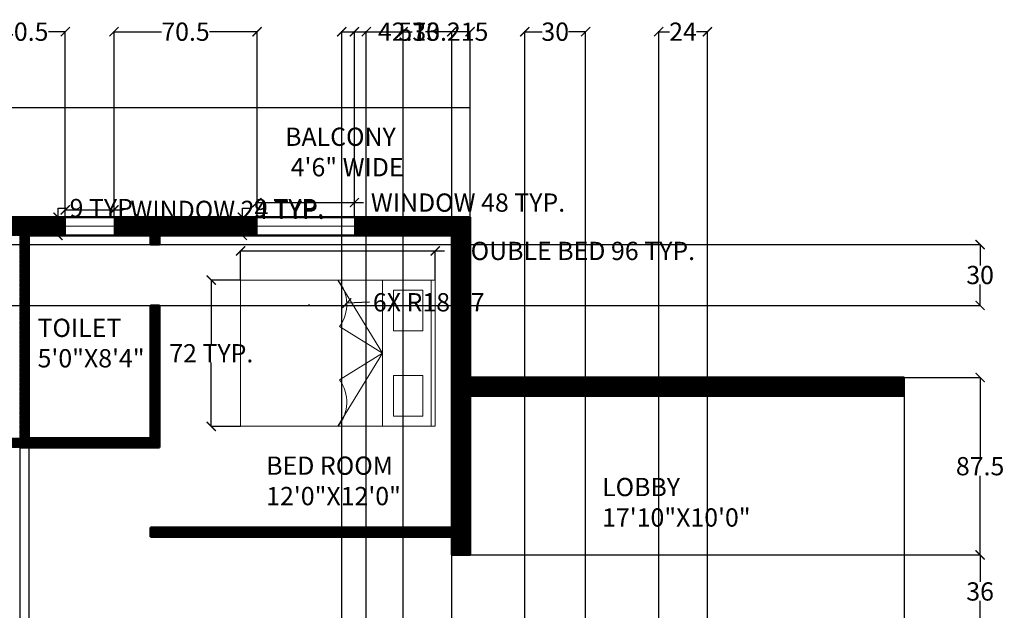
# Model space of a CAD drawing. Units: inches. Extents: x 273 to 1105, y 406 to 1027.
# Tile 3 of 3: x 612 to 1098, y 736 to 1027. Entities that reach past the tile are written whole.
import ezdxf

# ---------------------------------------------------------------- set-up
doc = ezdxf.new("R2010")
doc.units = ezdxf.units.IN
doc.header["$MEASUREMENT"] = 0
for name, color, linetype, lineweight in [('A-ANNO-DIMS', 2, 'Continuous', 18), ('A-AREA-IDEN', 7, 'Continuous', 18), ('A-FLOR-OTLN', 7, 'Continuous', 25), ('A-FURN', 8, 'Continuous', 18), ('A-GLAZ', 4, 'Continuous', 18), ('A-WALL', 7, 'Continuous', 50), ('A-WALL-PATT', 252, 'Continuous', 13)]:
    doc.layers.add(name, color=color, linetype=linetype, lineweight=lineweight)
doc.styles.get("Standard").update_dxf_attribs({"font": 'arial.ttf'})
doc.dimstyles.get("Standard").update_dxf_attribs({"dimtxt": 9, "dimasz": 4.5, "dimexe": 0.18, "dimexo": 0.0625, "dimgap": 0.09, "dimtad": 0, "dimtih": 1, "dimtoh": 1, "dimdec": 1, "dimzin": 0, "dimdsep": 46, "dimlunit": 4, "dimtxsty": 'Standard', "dimblk": 'ARCHTICK', "dimcen": 0.09, "dimadec": 0, "dimazin": 0, "dimtfac": 1, "dimtdec": 1, "dimtofl": 0, "dimtmove": 0, "dimatfit": 3, "dimfxl": 1, "dimtolj": 1, "dimtzin": 0, "dimarcsym": 0})

# ---------------------------------------------------------------- blocks, each defined once
blk = doc.blocks.new('BED-DOUBLE-72x96')
for p, q in [((0, 0.12), (0, 72.12)), ((0, 72.12), (96, 72.12)), ((48, 72.12), (70, 36.12)), ((70, 72.12), (70, 0.12)), ((94, 72.12), (94, 0.12)), ((96, 72.12), (96, 0.12)), ((48.84, 49.19), (70, 36.12)), ((70, 36.12), (48, 0.12)), ((70, 36.12), (48.84, 22.93)), ((96, 0.12), (0, 0.12))]:
    blk.add_line(p, q)
for points in [[(75.45, 67.24), (89.85, 67.24), (89.85, 47.07), (75.45, 47.07)], [(75.45, 5), (89.85, 5), (89.85, 25.18), (75.45, 25.18)]]:
    blk.add_lwpolyline(points, close=True)
for centre, start, end in [((33.83, 60.12), 323.9297, 40.2519), ((33.83, 12), 319.7481, 36.0703)]:
    blk.add_arc(centre, 18.57, start, end)
blk = doc.blocks.new('WIN-48')
for p, q in [((0, 9), (48, 9)), ((0, 0), (0, 9)), ((48, 9), (48, 0)), ((0, 4.5), (48, 4.5)), ((48, 0), (0, 0))]:
    blk.add_line(p, q)
blk = doc.blocks.new('WIN-24')
for p, q in [((0, 9), (24, 9)), ((0, 0), (0, 9)), ((24, 9), (24, 0)), ((0, 4.5), (24, 4.5)), ((24, 0), (0, 0))]:
    blk.add_line(p, q)
blk = doc.blocks.new('_ArchTick')
at = {"color": 0, "linetype": 'ByBlock', "const_width": 0.15}
blk.add_lwpolyline([(-0.5, -0.5), (0.5, 0.5)], dxfattribs=at)
blk = doc.blocks.new('*D6')
at = {"layer": 'A-ANNO-DIMS', "color": 0, "lineweight": -2, "transparency": 16777216}
for p, q in [((721.23, 898.64), (721.23, 913.15)), ((721.23, 912.97), (817.23, 912.97)), ((817.23, 898.64), (817.23, 913.15)), ((817.23, 912.97), (821.73, 912.97))]:
    blk.add_line(p, q, dxfattribs=at)
at = {"layer": 'Defpoints', "color": 0, "transparency": 16777216}
for p in [(817.23, 912.97), (721.23, 898.57), (817.23, 898.57)]:
    blk.add_point(p, dxfattribs=at)
at = {"layer": 'A-ANNO-DIMS', "color": 0, "lineweight": -2, "transparency": 16777216, "xscale": 4.5, "yscale": 4.5, "zscale": 4.5, "rotation": 180}
blk.add_blockref('_ArchTick', (721.23, 912.97), dxfattribs=at)
at = {"layer": 'A-ANNO-DIMS', "color": 0, "lineweight": -2, "transparency": 16777216, "xscale": 4.5, "yscale": 4.5, "zscale": 4.5}
blk.add_blockref('_ArchTick', (817.23, 912.97), dxfattribs=at)
at = {"layer": 'A-ANNO-DIMS', "color": 0, "transparency": 16777216, "insert": (885.77, 912.97), "char_height": 9, "attachment_point": 5}
blk.add_mtext('\\A1;DOUBLE BED 96 TYP.', dxfattribs=at)
blk = doc.blocks.new('*D7')
at = {"layer": 'A-ANNO-DIMS', "color": 0, "lineweight": -2, "transparency": 16777216}
for p, q in [((721.17, 898.57), (706.65, 898.57)), ((706.83, 898.57), (706.83, 867.12)), ((706.83, 826.45), (706.83, 857.9)), ((721.17, 826.45), (706.65, 826.45))]:
    blk.add_line(p, q, dxfattribs=at)
at = {"layer": 'Defpoints', "color": 0, "transparency": 16777216}
for p in [(706.83, 898.57), (721.23, 898.57), (721.23, 826.45)]:
    blk.add_point(p, dxfattribs=at)
at = {"layer": 'A-ANNO-DIMS', "color": 0, "lineweight": -2, "transparency": 16777216, "xscale": 4.5, "yscale": 4.5, "zscale": 4.5}
for p, rotation in [((706.83, 898.57), 90), ((706.83, 826.45), 270)]:
    blk.add_blockref('_ArchTick', p, dxfattribs=dict(at, rotation=rotation))
at = {"layer": 'A-ANNO-DIMS', "color": 0, "transparency": 16777216, "insert": (706.83, 862.51), "char_height": 9, "attachment_point": 5}
blk.add_mtext('\\A1;72 TYP.', dxfattribs=at)
blk = doc.blocks.new('*D8')
at = {"layer": 'A-ANNO-DIMS', "color": 0, "lineweight": -2, "transparency": 16777216}
for p, q in [((729.37, 929.67), (729.37, 936.98)), ((729.37, 936.8), (777.37, 936.8)), ((777.37, 929.67), (777.37, 936.98)), ((777.37, 936.8), (781.87, 936.8))]:
    blk.add_line(p, q, dxfattribs=at)
at = {"layer": 'Defpoints', "color": 0, "transparency": 16777216}
for p in [(777.37, 936.8), (729.37, 929.6), (777.37, 929.6)]:
    blk.add_point(p, dxfattribs=at)
at = {"layer": 'A-ANNO-DIMS', "color": 0, "lineweight": -2, "transparency": 16777216, "xscale": 4.5, "yscale": 4.5, "zscale": 4.5, "rotation": 180}
blk.add_blockref('_ArchTick', (729.37, 936.8), dxfattribs=at)
at = {"layer": 'A-ANNO-DIMS', "color": 0, "lineweight": -2, "transparency": 16777216, "xscale": 4.5, "yscale": 4.5, "zscale": 4.5}
blk.add_blockref('_ArchTick', (777.37, 936.8), dxfattribs=at)
at = {"layer": 'A-ANNO-DIMS', "color": 0, "transparency": 16777216, "insert": (833.38, 936.8), "char_height": 9, "attachment_point": 5}
blk.add_mtext('\\A1;WINDOW 48 TYP.', dxfattribs=at)
blk = doc.blocks.new('*D9')
at = {"layer": 'A-ANNO-DIMS', "color": 0, "lineweight": -2, "transparency": 16777216}
for p, q in [((722.17, 929.6), (722.17, 934.1)), ((722.17, 934.1), (726.67, 934.1)), ((729.31, 929.6), (721.99, 929.6)), ((722.17, 920.6), (722.17, 929.6)), ((729.31, 920.6), (721.99, 920.6))]:
    blk.add_line(p, q, dxfattribs=at)
at = {"layer": 'Defpoints', "color": 0, "transparency": 16777216}
for p in [(722.17, 929.6), (729.37, 929.6), (729.37, 920.6)]:
    blk.add_point(p, dxfattribs=at)
at = {"layer": 'A-ANNO-DIMS', "color": 0, "lineweight": -2, "transparency": 16777216, "xscale": 4.5, "yscale": 4.5, "zscale": 4.5}
for p, rotation in [((722.17, 929.6), 90), ((722.17, 920.6), 270)]:
    blk.add_blockref('_ArchTick', p, dxfattribs=dict(at, rotation=rotation))
at = {"layer": 'A-ANNO-DIMS', "color": 0, "transparency": 16777216, "insert": (745.17, 934.1), "char_height": 9, "attachment_point": 5}
blk.add_mtext('\\A1;9 TYP.', dxfattribs=at)
blk = doc.blocks.new('*D10')
at = {"layer": 'A-ANNO-DIMS', "color": 0, "lineweight": -2, "transparency": 16777216}
for p, q in [((634.87, 929.67), (634.87, 933.38)), ((634.87, 933.2), (658.87, 933.2)), ((658.87, 929.67), (658.87, 933.38)), ((658.87, 933.2), (663.37, 933.2))]:
    blk.add_line(p, q, dxfattribs=at)
at = {"layer": 'Defpoints', "color": 0, "transparency": 16777216}
for p in [(658.87, 933.2), (634.87, 929.6), (658.87, 929.6)]:
    blk.add_point(p, dxfattribs=at)
at = {"layer": 'A-ANNO-DIMS', "color": 0, "lineweight": -2, "transparency": 16777216, "xscale": 4.5, "yscale": 4.5, "zscale": 4.5, "rotation": 180}
blk.add_blockref('_ArchTick', (634.87, 933.2), dxfattribs=at)
at = {"layer": 'A-ANNO-DIMS', "color": 0, "lineweight": -2, "transparency": 16777216, "xscale": 4.5, "yscale": 4.5, "zscale": 4.5}
blk.add_blockref('_ArchTick', (658.87, 933.2), dxfattribs=at)
at = {"layer": 'A-ANNO-DIMS', "color": 0, "transparency": 16777216, "insert": (714.88, 933.2), "char_height": 9, "attachment_point": 5}
blk.add_mtext('\\A1;WINDOW 24 TYP.', dxfattribs=at)
blk = doc.blocks.new('*D11')
at = {"layer": 'A-ANNO-DIMS', "color": 0, "lineweight": -2, "transparency": 16777216}
for p, q in [((631.27, 929.6), (631.27, 934.1)), ((631.27, 934.1), (635.77, 934.1)), ((634.81, 929.6), (631.09, 929.6)), ((631.27, 920.6), (631.27, 929.6)), ((634.81, 920.6), (631.09, 920.6))]:
    blk.add_line(p, q, dxfattribs=at)
at = {"layer": 'Defpoints', "color": 0, "transparency": 16777216}
for p in [(631.27, 929.6), (634.87, 929.6), (634.87, 920.6)]:
    blk.add_point(p, dxfattribs=at)
at = {"layer": 'A-ANNO-DIMS', "color": 0, "lineweight": -2, "transparency": 16777216, "xscale": 4.5, "yscale": 4.5, "zscale": 4.5}
for p, rotation in [((631.27, 929.6), 90), ((631.27, 920.6), 270)]:
    blk.add_blockref('_ArchTick', p, dxfattribs=dict(at, rotation=rotation))
at = {"layer": 'A-ANNO-DIMS', "color": 0, "transparency": 16777216, "insert": (654.27, 934.1), "char_height": 9, "attachment_point": 5}
blk.add_mtext('\\A1;9 TYP.', dxfattribs=at)
blk = doc.blocks.new('*D19')
at = {"layer": 'A-ANNO-DIMS', "color": 0, "lineweight": -2, "transparency": 16777216}
for p, q in [((594.37, 929.67), (594.37, 1021.23)), ((594.37, 1021.05), (602.63, 1021.05)), ((634.87, 1021.05), (626.62, 1021.05)), ((634.87, 929.67), (634.87, 1021.23))]:
    blk.add_line(p, q, dxfattribs=at)
at = {"layer": 'Defpoints', "color": 0, "transparency": 16777216}
for p in [(634.87, 1021.05), (594.37, 929.6), (634.87, 929.6)]:
    blk.add_point(p, dxfattribs=at)
at = {"layer": 'A-ANNO-DIMS', "color": 0, "lineweight": -2, "transparency": 16777216, "xscale": 4.5, "yscale": 4.5, "zscale": 4.5, "rotation": 180}
blk.add_blockref('_ArchTick', (594.37, 1021.05), dxfattribs=at)
at = {"layer": 'A-ANNO-DIMS', "color": 0, "lineweight": -2, "transparency": 16777216, "xscale": 4.5, "yscale": 4.5, "zscale": 4.5}
blk.add_blockref('_ArchTick', (634.87, 1021.05), dxfattribs=at)
at = {"layer": 'A-ANNO-DIMS', "color": 0, "transparency": 16777216, "insert": (614.62, 1021.05), "char_height": 9, "attachment_point": 5}
blk.add_mtext('\\A1;40.5', dxfattribs=at)
blk = doc.blocks.new('*D20')
at = {"layer": 'A-ANNO-DIMS', "color": 0, "lineweight": -2, "transparency": 16777216}
for p, q in [((658.87, 929.67), (658.87, 1021.23)), ((658.87, 1021.05), (682.35, 1021.05)), ((729.37, 1021.05), (705.9, 1021.05)), ((729.37, 929.67), (729.37, 1021.23))]:
    blk.add_line(p, q, dxfattribs=at)
at = {"layer": 'Defpoints', "color": 0, "transparency": 16777216}
for p in [(729.37, 1021.05), (658.87, 929.6), (729.37, 929.6)]:
    blk.add_point(p, dxfattribs=at)
at = {"layer": 'A-ANNO-DIMS', "color": 0, "lineweight": -2, "transparency": 16777216, "xscale": 4.5, "yscale": 4.5, "zscale": 4.5, "rotation": 180}
blk.add_blockref('_ArchTick', (658.87, 1021.05), dxfattribs=at)
at = {"layer": 'A-ANNO-DIMS', "color": 0, "lineweight": -2, "transparency": 16777216, "xscale": 4.5, "yscale": 4.5, "zscale": 4.5}
blk.add_blockref('_ArchTick', (729.37, 1021.05), dxfattribs=at)
at = {"layer": 'A-ANNO-DIMS', "color": 0, "transparency": 16777216, "insert": (694.12, 1021.05), "char_height": 9, "attachment_point": 5}
blk.add_mtext('\\A1;70.5', dxfattribs=at)
blk = doc.blocks.new('*D21')
at = {"layer": 'A-ANNO-DIMS', "color": 0, "lineweight": -2, "transparency": 16777216}
for p, q in [((777.37, 929.67), (777.37, 1021.23)), ((777.37, 1021.05), (799.34, 1021.05)), ((834.37, 1021.05), (812.41, 1021.05)), ((834.37, 929.67), (834.37, 1021.23))]:
    blk.add_line(p, q, dxfattribs=at)
at = {"layer": 'Defpoints', "color": 0, "transparency": 16777216}
for p in [(834.37, 1021.05), (777.37, 929.6), (834.37, 929.6)]:
    blk.add_point(p, dxfattribs=at)
at = {"layer": 'A-ANNO-DIMS', "color": 0, "lineweight": -2, "transparency": 16777216, "xscale": 4.5, "yscale": 4.5, "zscale": 4.5, "rotation": 180}
blk.add_blockref('_ArchTick', (777.37, 1021.05), dxfattribs=at)
at = {"layer": 'A-ANNO-DIMS', "color": 0, "lineweight": -2, "transparency": 16777216, "xscale": 4.5, "yscale": 4.5, "zscale": 4.5}
blk.add_blockref('_ArchTick', (834.37, 1021.05), dxfattribs=at)
at = {"layer": 'A-ANNO-DIMS', "color": 0, "transparency": 16777216, "insert": (805.87, 1021.05), "char_height": 9, "attachment_point": 5}
blk.add_mtext('\\A1;57', dxfattribs=at)
blk = doc.blocks.new('*D23')
at = {"layer": 'A-ANNO-DIMS', "color": 0, "lineweight": -2, "transparency": 16777216}
for p, q in [((834.44, 763.1), (1086, 763.1)), ((1085.82, 763.1), (1085.82, 749.79)), ((1085.82, 727.1), (1085.82, 740.42)), ((960.44, 727.1), (1086, 727.1))]:
    blk.add_line(p, q, dxfattribs=at)
at = {"layer": 'Defpoints', "color": 0, "transparency": 16777216}
for p in [(834.37, 763.1), (1085.82, 763.1), (960.37, 727.1)]:
    blk.add_point(p, dxfattribs=at)
at = {"layer": 'A-ANNO-DIMS', "color": 0, "lineweight": -2, "transparency": 16777216, "xscale": 4.5, "yscale": 4.5, "zscale": 4.5}
for p, rotation in [((1085.82, 763.1), 90), ((1085.82, 727.1), 270)]:
    blk.add_blockref('_ArchTick', p, dxfattribs=dict(at, rotation=rotation))
at = {"layer": 'A-ANNO-DIMS', "color": 0, "transparency": 16777216, "insert": (1085.82, 745.1), "char_height": 9, "attachment_point": 5}
blk.add_mtext('\\A1;36', dxfattribs=at)
blk = doc.blocks.new('*D24')
at = {"layer": 'A-ANNO-DIMS', "color": 0, "lineweight": -2, "transparency": 16777216}
for p, q in [((1048.44, 850.6), (1086, 850.6)), ((1085.82, 850.6), (1085.82, 811.54)), ((1085.82, 763.1), (1085.82, 802.17)), ((834.44, 763.1), (1086, 763.1))]:
    blk.add_line(p, q, dxfattribs=at)
at = {"layer": 'Defpoints', "color": 0, "transparency": 16777216}
for p in [(1048.37, 850.6), (1085.82, 850.6), (834.37, 763.1)]:
    blk.add_point(p, dxfattribs=at)
at = {"layer": 'A-ANNO-DIMS', "color": 0, "lineweight": -2, "transparency": 16777216, "xscale": 4.5, "yscale": 4.5, "zscale": 4.5}
for p, rotation in [((1085.82, 850.6), 90), ((1085.82, 763.1), 270)]:
    blk.add_blockref('_ArchTick', p, dxfattribs=dict(at, rotation=rotation))
at = {"layer": 'A-ANNO-DIMS', "color": 0, "transparency": 16777216, "insert": (1085.82, 806.85), "char_height": 9, "attachment_point": 5}
blk.add_mtext('\\A1;87.5', dxfattribs=at)
blk = doc.blocks.new('*D25')
at = {"layer": 'A-ANNO-DIMS', "color": 0, "lineweight": -2, "transparency": 16777216}
for p, q in [((927.37, 721.67), (927.37, 1021.23)), ((927.37, 1021.05), (932.78, 1021.05)), ((951.37, 1021.05), (945.97, 1021.05)), ((951.37, 721.67), (951.37, 1021.23))]:
    blk.add_line(p, q, dxfattribs=at)
at = {"layer": 'Defpoints', "color": 0, "transparency": 16777216}
for p in [(951.37, 1021.05), (927.37, 721.6), (951.37, 721.6)]:
    blk.add_point(p, dxfattribs=at)
at = {"layer": 'A-ANNO-DIMS', "color": 0, "lineweight": -2, "transparency": 16777216, "xscale": 4.5, "yscale": 4.5, "zscale": 4.5, "rotation": 180}
blk.add_blockref('_ArchTick', (927.37, 1021.05), dxfattribs=at)
at = {"layer": 'A-ANNO-DIMS', "color": 0, "lineweight": -2, "transparency": 16777216, "xscale": 4.5, "yscale": 4.5, "zscale": 4.5}
blk.add_blockref('_ArchTick', (951.37, 1021.05), dxfattribs=at)
at = {"layer": 'A-ANNO-DIMS', "color": 0, "transparency": 16777216, "insert": (939.37, 1021.05), "char_height": 9, "attachment_point": 5}
blk.add_mtext('\\A1;24', dxfattribs=at)
blk = doc.blocks.new('*D26')
at = {"layer": 'A-ANNO-DIMS', "color": 0, "lineweight": -2, "transparency": 16777216}
for p, q in [((861.37, 592.67), (861.37, 1021.23)), ((861.37, 1021.05), (869.86, 1021.05)), ((891.37, 1021.05), (882.89, 1021.05)), ((891.37, 592.67), (891.37, 1021.23))]:
    blk.add_line(p, q, dxfattribs=at)
at = {"layer": 'Defpoints', "color": 0, "transparency": 16777216}
for p in [(891.37, 1021.05), (861.37, 592.6), (891.37, 592.6)]:
    blk.add_point(p, dxfattribs=at)
at = {"layer": 'A-ANNO-DIMS', "color": 0, "lineweight": -2, "transparency": 16777216, "xscale": 4.5, "yscale": 4.5, "zscale": 4.5, "rotation": 180}
blk.add_blockref('_ArchTick', (861.37, 1021.05), dxfattribs=at)
at = {"layer": 'A-ANNO-DIMS', "color": 0, "lineweight": -2, "transparency": 16777216, "xscale": 4.5, "yscale": 4.5, "zscale": 4.5}
blk.add_blockref('_ArchTick', (891.37, 1021.05), dxfattribs=at)
at = {"layer": 'A-ANNO-DIMS', "color": 0, "transparency": 16777216, "insert": (876.37, 1021.05), "char_height": 9, "attachment_point": 5}
blk.add_mtext('\\A1;30', dxfattribs=at)
blk = doc.blocks.new('*D28')
at = {"layer": 'A-ANNO-DIMS', "color": 0, "lineweight": -2, "transparency": 16777216}
for p, q in [((783.25, 481.67), (783.25, 1021.23)), ((783.25, 1021.05), (788.85, 1021.05)), ((825.37, 1021.05), (819.77, 1021.05)), ((825.37, 481.67), (825.37, 1021.23))]:
    blk.add_line(p, q, dxfattribs=at)
at = {"layer": 'Defpoints', "color": 0, "transparency": 16777216}
for p in [(825.37, 1021.05), (783.25, 481.6), (825.37, 481.6)]:
    blk.add_point(p, dxfattribs=at)
at = {"layer": 'A-ANNO-DIMS', "color": 0, "lineweight": -2, "transparency": 16777216, "xscale": 4.5, "yscale": 4.5, "zscale": 4.5, "rotation": 180}
blk.add_blockref('_ArchTick', (783.25, 1021.05), dxfattribs=at)
at = {"layer": 'A-ANNO-DIMS', "color": 0, "lineweight": -2, "transparency": 16777216, "xscale": 4.5, "yscale": 4.5, "zscale": 4.5}
blk.add_blockref('_ArchTick', (825.37, 1021.05), dxfattribs=at)
at = {"layer": 'A-ANNO-DIMS', "color": 0, "transparency": 16777216, "insert": (804.31, 1021.05), "char_height": 9, "attachment_point": 5}
blk.add_mtext('\\A1;42.13', dxfattribs=at)
blk = doc.blocks.new('*D30')
at = {"layer": 'A-ANNO-DIMS', "color": 0, "lineweight": -2, "transparency": 16777216}
for p, q in [((552.44, 916.1), (1086, 916.1)), ((1085.82, 916.1), (1085.82, 905.79)), ((1085.82, 886.1), (1085.82, 896.42)), ((552.44, 886.1), (1086, 886.1))]:
    blk.add_line(p, q, dxfattribs=at)
at = {"layer": 'Defpoints', "color": 0, "transparency": 16777216}
for p in [(552.37, 916.1), (552.37, 886.1), (1085.82, 886.1)]:
    blk.add_point(p, dxfattribs=at)
at = {"layer": 'A-ANNO-DIMS', "color": 0, "lineweight": -2, "transparency": 16777216, "xscale": 4.5, "yscale": 4.5, "zscale": 4.5}
for p, rotation in [((1085.82, 916.1), 90), ((1085.82, 886.1), 270)]:
    blk.add_blockref('_ArchTick', p, dxfattribs=dict(at, rotation=rotation))
at = {"layer": 'A-ANNO-DIMS', "color": 0, "transparency": 16777216, "insert": (1085.82, 901.1), "char_height": 9, "attachment_point": 5}
blk.add_mtext('\\A1;30', dxfattribs=at)
blk = doc.blocks.new('*D31')
at = {"layer": 'A-ANNO-DIMS', "color": 0, "lineweight": -2, "transparency": 16777216}
for p, q in [((612.37, 820.54), (612.37, 434.97)), ((616.87, 820.54), (616.87, 434.97)), ((612.37, 435.15), (616.87, 435.15)), ((616.87, 435.15), (621.37, 435.15))]:
    blk.add_line(p, q, dxfattribs=at)
at = {"layer": 'Defpoints', "color": 0, "transparency": 16777216}
for p in [(612.37, 820.6), (616.87, 820.6), (616.87, 435.15)]:
    blk.add_point(p, dxfattribs=at)
at = {"layer": 'A-ANNO-DIMS', "color": 0, "lineweight": -2, "transparency": 16777216, "xscale": 4.5, "yscale": 4.5, "zscale": 4.5, "rotation": 180}
blk.add_blockref('_ArchTick', (612.37, 435.15), dxfattribs=at)
at = {"layer": 'A-ANNO-DIMS', "color": 0, "lineweight": -2, "transparency": 16777216, "xscale": 4.5, "yscale": 4.5, "zscale": 4.5}
blk.add_blockref('_ArchTick', (616.87, 435.15), dxfattribs=at)
at = {"layer": 'A-ANNO-DIMS', "color": 0, "transparency": 16777216, "insert": (629.87, 435.15), "char_height": 9, "attachment_point": 5}
blk.add_mtext('\\A1;4.5', dxfattribs=at)
blk = doc.blocks.new('*D38')
at = {"layer": 'A-ANNO-DIMS', "color": 0, "lineweight": -2, "transparency": 16777216}
for p, q in [((771.16, 560.63), (771.16, 1021.23)), ((771.16, 1021.05), (801.37, 1021.05)), ((801.37, 564.17), (801.37, 1021.23)), ((801.37, 1021.05), (805.87, 1021.05))]:
    blk.add_line(p, q, dxfattribs=at)
at = {"layer": 'Defpoints', "color": 0, "transparency": 16777216}
for p in [(801.37, 1021.05), (801.37, 564.1), (771.16, 560.57)]:
    blk.add_point(p, dxfattribs=at)
at = {"layer": 'A-ANNO-DIMS', "color": 0, "lineweight": -2, "transparency": 16777216, "xscale": 4.5, "yscale": 4.5, "zscale": 4.5, "rotation": 180}
blk.add_blockref('_ArchTick', (771.16, 1021.05), dxfattribs=at)
at = {"layer": 'A-ANNO-DIMS', "color": 0, "lineweight": -2, "transparency": 16777216, "xscale": 4.5, "yscale": 4.5, "zscale": 4.5}
blk.add_blockref('_ArchTick', (801.37, 1021.05), dxfattribs=at)
at = {"layer": 'A-ANNO-DIMS', "color": 0, "transparency": 16777216, "insert": (824.68, 1021.05), "char_height": 9, "attachment_point": 5}
blk.add_mtext('\\A1;30.215', dxfattribs=at)
blk = doc.blocks.new('*D40')
at = {"layer": 'A-ANNO-DIMS', "color": 0, "lineweight": -2, "transparency": 16777216}
for p, q in [((754.97, 886.57), (755.15, 886.57)), ((755.06, 886.48), (755.06, 886.66)), ((784.75, 887.66), (773.62, 887.25))]:
    blk.add_line(p, q, dxfattribs=at)
at = {"layer": 'Defpoints', "color": 0, "transparency": 16777216}
for p in [(755.06, 886.57), (773.62, 887.25)]:
    blk.add_point(p, dxfattribs=at)
at = {"layer": 'A-ANNO-DIMS', "color": 0, "lineweight": -2, "transparency": 16777216, "xscale": 4.5, "yscale": 4.5, "zscale": 4.5, "rotation": 182.0894062445447}
blk.add_blockref('_ArchTick', (773.62, 887.25), dxfattribs=at)
at = {"layer": 'A-ANNO-DIMS', "color": 0, "transparency": 16777216, "insert": (814.03, 887.66), "char_height": 9, "attachment_point": 5}
blk.add_mtext('\\A1;6X R18.57', dxfattribs=at)

msp = doc.modelspace()

# ---------------------------------------------------------------- hatches: boundary and pattern name
at = {"layer": 'A-WALL-PATT'}
h = msp.add_hatch(dxfattribs=at)
h.set_pattern_fill('ANSI31', color=256)
h.paths.add_polyline_path([(735.2471, 481.6046), (681.3741, 481.6046), (681.3741, 535.6046), (825.3741, 535.6046), (825.3741, 481.6046), (783.2471, 481.6046), (783.2471, 472.6046), (834.3741, 472.6046), (834.3741, 592.6046), (861.3741, 592.6046), (861.3741, 601.6046), (834.3741, 601.6046), (834.3741, 721.6046), (918.3741, 721.6046), (918.3741, 601.6046), (891.3741, 601.6046), (891.3741, 592.6046), (960.3741, 592.6046), (960.3741, 617.3546), (951.3741, 617.3546), (951.3741, 601.6046), (927.3741, 601.6046), (927.3741, 657.1046), (951.3741, 657.1046), (951.3741, 641.3546), (960.3741, 641.3546), (960.3741, 681.8546), (951.3741, 681.8546), (951.3741, 666.1046), (927.3741, 666.1046), (927.3741, 721.6046), (951.3741, 721.6046), (951.3741, 705.8546), (960.3741, 705.8546), (960.3741, 727.1046), (834.3741, 727.1046), (825.3741, 727.1046), (825.3741, 640.1046), (681.3741, 640.1046), (676.8741, 640.1046), (676.8741, 635.6046), (681.3741, 635.6046), (825.3741, 635.6046), (825.3741, 540.1046), (681.3741, 540.1046), (681.3741, 588.1046), (676.8741, 588.1046), (616.8741, 588.1046), (616.8741, 644.6046), (612.3741, 644.6046), (612.3741, 640.1046), (612.3741, 588.1046), (552.3741, 588.1046), (552.3741, 640.1046), (552.3741, 644.6046), (547.8741, 644.6046), (547.8741, 640.1046), (547.8741, 635.6046), (547.8741, 547.6046), (552.3741, 547.6046), (552.3741, 583.6046), (602.3741, 583.6046), (602.3741, 547.6046), (606.8741, 547.6046), (606.8741, 583.6046), (676.8741, 583.6046), (676.8741, 481.6046), (552.3741, 481.6046), (552.3741, 517.6046), (547.8741, 517.6046), (547.8741, 481.6046), (493.8741, 481.6046), (493.8741, 472.6046), (547.8741, 472.6046), (735.2471, 472.6046)])
h.paths.add_polyline_path([(445.8741, 481.6046), (391.8741, 481.6046), (391.8741, 576.6354), (382.8741, 576.6354), (382.8741, 472.6046), (391.8741, 472.6046), (445.8741, 472.6046)])
h.paths.add_polyline_path([(729.3741, 929.6046), (658.8741, 929.6046), (658.8741, 920.6046), (676.8741, 920.6046), (676.8741, 916.1046), (681.3741, 916.1046), (681.3741, 920.6046), (729.3741, 920.6046)])
h.paths.add_polyline_path([(834.3741, 929.6046), (777.3741, 929.6046), (777.3741, 920.6046), (825.3741, 920.6046), (825.3741, 776.6046), (681.3741, 776.6046), (676.8741, 776.6046), (676.8741, 772.1046), (681.3741, 772.1046), (825.3741, 772.1046), (825.3741, 763.1046), (834.3741, 763.1046)])
h.paths.add_polyline_path([(1048.3741, 850.6046), (834.3741, 850.6046), (834.3741, 841.6046), (1048.3741, 841.6046)])
h.paths.add_polyline_path([(337.8741, 772.1046), (391.8741, 772.1046), (415.8741, 772.1046), (420.3741, 772.1046), (424.8741, 772.1046), (547.8741, 772.1046), (547.8741, 774.3546), (424.8741, 774.3546), (424.8741, 776.6046), (391.8741, 776.6046), (391.8741, 920.6046), (445.8741, 920.6046), (445.8741, 929.6046), (382.8741, 929.6046), (382.8741, 776.6046), (328.8741, 776.6046), (328.8741, 772.1046), (328.8741, 635.6046), (382.8741, 635.6046), (391.8741, 635.6046), (424.8741, 635.6046), (511.8741, 635.6046), (511.8741, 640.1046), (415.8741, 640.1046), (391.8741, 640.1046), (337.8741, 640.1046)])
h.paths.add_polyline_path([(570.3741, 929.6046), (493.8741, 929.6046), (493.8741, 920.6046), (547.8741, 920.6046), (547.8741, 916.1046), (552.3741, 916.1046), (552.3741, 920.6046), (570.3741, 920.6046)])
h.paths.add_polyline_path([(634.8741, 929.6046), (594.3741, 929.6046), (594.3741, 920.6046), (612.3741, 920.6046), (612.3741, 820.6046), (552.3741, 820.6046), (552.3741, 886.1046), (547.8741, 886.1046), (547.8741, 816.1046), (552.3741, 816.1046), (612.3741, 816.1046), (616.8741, 816.1046), (676.8741, 816.1046), (681.3741, 816.1046), (681.3741, 886.1046), (676.8741, 886.1046), (676.8741, 820.6046), (616.8741, 820.6046), (616.8741, 920.6046), (634.8741, 920.6046)])

# ---------------------------------------------------------------- linework, layer by layer
at = {"layer": 'A-FLOR-OTLN'}
for p, q in [((382.8741, 983.6046), (834.3741, 983.6046)), ((834.3741, 929.6046), (834.3741, 983.6046)), ((1048.3741, 850.6046), (1048.3741, 763.1046)), ((1048.3741, 763.1046), (1048.3741, 724.6658))]:
    msp.add_line(p, q, dxfattribs=at)
at = {"layer": 'A-WALL'}
for p, q in [((382.8741, 929.6046), (834.3741, 929.6046)), ((834.3741, 929.6046), (834.3741, 763.1046)), ((616.8741, 920.6046), (616.8741, 820.6046)), ((616.8741, 920.6046), (676.8741, 920.6046)), ((676.8741, 920.6046), (676.8741, 916.1046)), ((681.3741, 920.6046), (681.3741, 916.1046)), ((681.3741, 920.6046), (825.3741, 920.6046)), ((825.3741, 920.6046), (825.3741, 776.6046)), ((676.8741, 916.1046), (681.3741, 916.1046)), ((676.8741, 886.1046), (681.3741, 886.1046)), ((676.8741, 886.1046), (676.8741, 820.6046)), ((681.3741, 886.1046), (681.3741, 816.1046)), ((834.3741, 850.6046), (1048.3741, 850.6046)), ((834.3741, 841.6046), (1048.3741, 841.6046)), ((616.8741, 820.6046), (676.8741, 820.6046)), ((612.3741, 816.1046), (616.8741, 816.1046)), ((616.8741, 816.1046), (676.8741, 816.1046)), ((676.8741, 816.1046), (681.3741, 816.1046)), ((676.8741, 776.6046), (676.8741, 772.1046)), ((681.3741, 776.6046), (676.8741, 776.6046)), ((681.3741, 772.1046), (676.8741, 772.1046)), ((681.3741, 776.6046), (825.3741, 776.6046)), ((681.3741, 772.1046), (825.3741, 772.1046)), ((825.3741, 772.1046), (825.3741, 763.1046)), ((825.3741, 763.1046), (834.3741, 763.1046))]:
    msp.add_line(p, q, dxfattribs=at)

# ---------------------------------------------------------------- block references
at = {"layer": 'A-FURN'}
msp.add_blockref('BED-DOUBLE-72x96', (721.233, 826.452), dxfattribs=at)
at = {"layer": 'A-GLAZ'}
for name, p in [('WIN-24', (634.874, 920.605)), ('WIN-48', (729.374, 920.605))]:
    msp.add_blockref(name, p, dxfattribs=at)

# ---------------------------------------------------------------- texts
at = {"layer": 'A-AREA-IDEN', "char_height": 9, "attachment_point": 1}
for s, insert in [('BALCONY\\P 4\'6" WIDE', (743.2301, 973.7535)), (' TOILET\\P 5\'0"X8\'4"', (618.441, 879.559)), ('BED ROOM\\P12\'0"X12\'0"', (733.9035, 811.6187)), ('LOBBY\\P17\'10"X10\'0"', (899.4765, 801.0769))]:
    msp.add_mtext_dynamic_manual_height_columns(s, width=435.167248, gutter_width=1, heights=[0], dxfattribs=dict(at, insert=insert))

# ---------------------------------------------------------------- dimensions: what is measured, and where the dimension line sits
at = {"layer": 'A-ANNO-DIMS'}
for base, p1, p2, override, picture, middle in [((634.8741, 1021.0546), (594.3741, 929.6046), (634.8741, 929.6046), {"dimdec": 1, "dimlfac": 1, "dimrnd": 0, "dimzin": 0, "dimdsep": 46, "dimlunit": 2}, '*D19', (614.6241, 1021.0546)), ((729.3741, 1021.0546), (658.8741, 929.6046), (729.3741, 929.6046), {"dimdec": 1, "dimlfac": 1, "dimrnd": 0, "dimzin": 0, "dimdsep": 46, "dimlunit": 2}, '*D20', (694.1241, 1021.0546)), ((801.37409, 1021.05461), (771.15955, 560.56745), (801.37409, 564.1046), {"dimdec": 3, "dimlfac": 1, "dimrnd": 0, "dimzin": 0, "dimdsep": 46, "dimlunit": 2}, '*D38', (824.67623, 1021.05461)), ((834.3741, 1021.0546), (777.3741, 929.6046), (834.3741, 929.6046), {"dimdec": 0, "dimlfac": 1, "dimrnd": 0, "dimzin": 0, "dimdsep": 46, "dimlunit": 2}, '*D21', (805.8741, 1021.0546)), ((825.3741, 1021.0546), (783.2471, 481.6046), (825.3741, 481.6046), {"dimdec": 2, "dimlfac": 1, "dimrnd": 0, "dimzin": 0, "dimdsep": 46, "dimlunit": 2}, '*D28', (804.3106, 1021.0546)), ((891.3741, 1021.0546), (861.3741, 592.6046), (891.3741, 592.6046), {"dimdec": 0, "dimlfac": 1, "dimrnd": 0, "dimzin": 0, "dimdsep": 46, "dimlunit": 2}, '*D26', (876.3741, 1021.0546)), ((951.3741, 1021.0546), (927.3741, 721.6046), (951.3741, 721.6046), {"dimdec": 0, "dimlfac": 1, "dimrnd": 0, "dimzin": 0, "dimdsep": 46, "dimlunit": 2}, '*D25', (939.3741, 1021.0546)), ((616.8741, 435.1546), (612.3741, 820.6046), (616.8741, 820.6046), {"dimdec": 1, "dimlfac": 1, "dimrnd": 0, "dimzin": 0, "dimdsep": 46, "dimlunit": 2}, '*D31', (629.8717, 435.1546))]:
    dim = msp.add_linear_dim(base=base, p1=p1, p2=p2, dimstyle='Standard', override=override, dxfattribs=at)
    dim.commit()
    dim.dimension.update_dxf_attribs({"geometry": picture, "text_midpoint": middle})
for base, p1, p2, text, picture, middle in [((777.3741, 936.8046), (729.3741, 929.6046), (777.3741, 929.6046), 'WINDOW <> TYP.', '*D8', (833.3826, 936.8046)), ((658.8741, 933.2046), (634.8741, 929.6046), (658.8741, 929.6046), 'WINDOW <> TYP.', '*D10', (714.8826, 933.2046)), ((817.2331, 912.9731), (721.2331, 898.5731), (817.2331, 898.5731), 'DOUBLE BED <> TYP.', '*D6', (885.7746, 912.9731))]:
    dim = msp.add_linear_dim(base=base, p1=p1, p2=p2, text=text, dimstyle='Standard', override={"dimdec": 0, "dimlfac": 1, "dimrnd": 0, "dimzin": 0, "dimdsep": 46, "dimlunit": 2}, dxfattribs=at)
    dim.commit()
    dim.dimension.update_dxf_attribs({"geometry": picture, "text_midpoint": middle})
for base, p1, p2, picture, middle in [((631.2741, 929.6046), (634.8741, 920.6046), (634.8741, 929.6046), '*D11', (654.2723, 934.1046)), ((722.1741, 929.6046), (729.3741, 920.6046), (729.3741, 929.6046), '*D9', (745.1723, 934.1046)), ((706.8331, 898.5731), (721.2331, 826.4523), (721.2331, 898.5731), '*D7', (706.8331, 862.5127))]:
    dim = msp.add_linear_dim(base=base, p1=p1, p2=p2, angle=90, text='<> TYP.', dimstyle='Standard', override={"dimdec": 0, "dimlfac": 1, "dimrnd": 0, "dimzin": 0, "dimdsep": 46, "dimlunit": 2}, dxfattribs=at)
    dim.commit()
    dim.dimension.update_dxf_attribs({"geometry": picture, "text_midpoint": middle})
for base, p1, p2, override, picture, middle in [((1085.8241, 886.1046), (552.3741, 916.1046), (552.3741, 886.1046), {"dimdec": 0, "dimlfac": 1, "dimrnd": 0, "dimzin": 0, "dimdsep": 46, "dimlunit": 2}, '*D30', (1085.8241, 901.1046)), ((1085.8241, 850.6046), (834.3741, 763.1046), (1048.3741, 850.6046), {"dimdec": 1, "dimlfac": 1, "dimrnd": 0, "dimzin": 0, "dimdsep": 46, "dimlunit": 2}, '*D24', (1085.8241, 806.8546)), ((1085.8241, 763.1046), (960.3741, 727.1046), (834.3741, 763.1046), {"dimdec": 0, "dimlfac": 1, "dimrnd": 0, "dimzin": 0, "dimdsep": 46, "dimlunit": 2}, '*D23', (1085.8241, 745.1046))]:
    dim = msp.add_linear_dim(base=base, p1=p1, p2=p2, angle=90, dimstyle='Standard', override=override, dxfattribs=at)
    dim.commit()
    dim.dimension.update_dxf_attribs({"geometry": picture, "text_midpoint": middle})
dim = msp.add_radius_dim(center=(755.0613, 886.575), mpoint=(773.6176, 887.252), text='6X <>', dimstyle='Standard', override={"dimdec": 2, "dimlfac": 1, "dimrnd": 0, "dimzin": 0, "dimdsep": 46, "dimlunit": 2}, dxfattribs=at)
dim.commit()
dim.dimension.update_dxf_attribs({"geometry": '*D40', "text_midpoint": (784.7513, 887.6582), "dimtype": 164})

doc.saveas('drawing.dxf')
